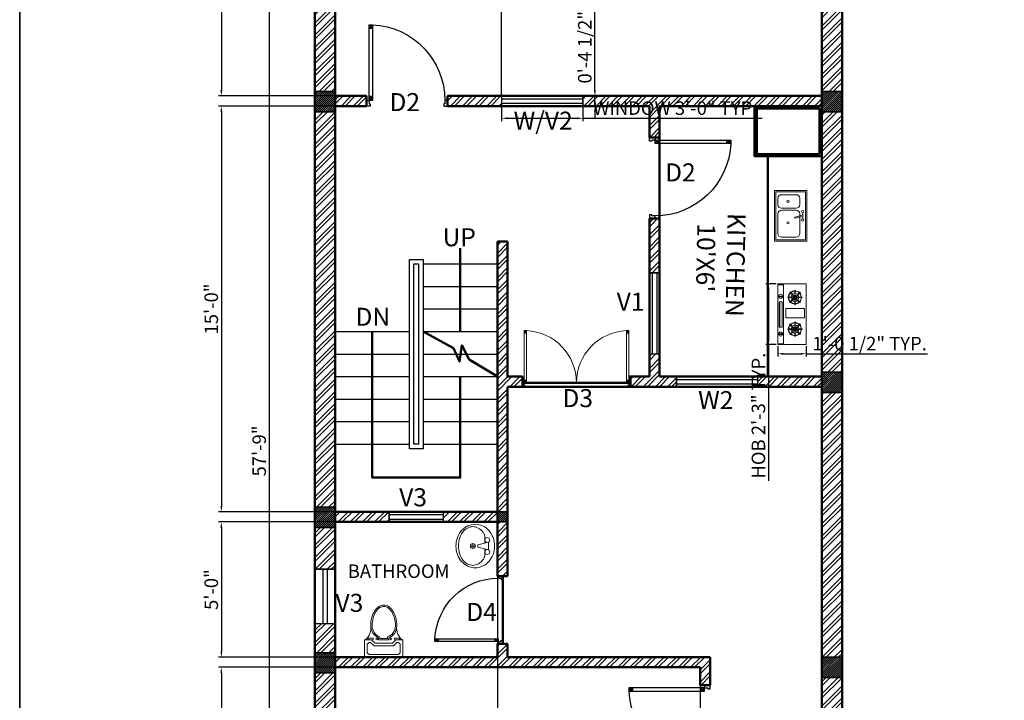
# Model space of a CAD drawing. Units: millimetres. Extents: x 20768 to 23556, y 50760 to 52704.
# Tile 20 of 36: x 20768 to 21205, y 52066 to 52368. Entities that reach past the tile are written whole.
import ezdxf

# ---------------------------------------------------------------- set-up
doc = ezdxf.new("R2010")
doc.units = ezdxf.units.MM
for name, color, linetype, lineweight in [('A-ANNO-DIMS', 2, 'Continuous', 18), ('A-ANNO-TTLB', 7, 'Continuous', 35), ('A-AREA-IDEN', 40, 'Continuous', 18), ('A-DOOR', 3, 'Continuous', 25), ('A-FLOR-STRS', 11, 'Continuous', 25), ('A-FURN', 8, 'Continuous', 18), ('A-GLAZ', 4, 'Continuous', 25), ('A-WALL', 7, 'Continuous', 50), ('A-WALL-PATT', 8, 'Continuous', 13), ('S-ANNO-DIMS', 2, 'Continuous', 18), ('S-COLS', 20, 'Continuous', 35)]:
    doc.layers.add(name, color=color, linetype=linetype, lineweight=lineweight)
doc.styles.get("Standard").update_dxf_attribs({"font": 'arial.ttf'})
doc.dimstyles.new('ISO-25', dxfattribs={"dimtxt": 6, "dimasz": 2.5, "dimexe": 1.25, "dimexo": 0.625, "dimtad": 1, "dimdec": 0, "dimlunit": 3, "dimtxsty": 'Standard', "dimcen": 2.5, "dimadec": 0, "dimazin": 0, "dimtfac": 1, "dimtdec": 0, "dimtmove": 0, "dimatfit": 3, "dimfxl": 1, "dimarcsym": 0})
pattern_1 = [(45, (-81.11126, 0), (-0.449012806, 0.449012806), [])]
pattern_2 = [(45, (-81.1113, 0), (-2.69407684, 2.69407684), []), (45, (-79.3152, 0), (-2.69407684, 2.69407684), [])]

# ---------------------------------------------------------------- blocks, each defined once
blk = doc.blocks.new('Puerta 01')
for p, q in [((-0.7745, -0.0264), (-0.7368, -0.0584)), ((-0.7745, -0.0584), (-0.7368, -0.0264)), ((-0.7368, -0.0584), (-0.7368, -0.0264)), ((-0.028, -0.0584), (-0.0657, -0.0264)), ((-0.028, -0.0264), (-0.0657, -0.0584)), ((-0.0657, -0.0584), (-0.0657, -0.0264))]:
    blk.add_line(p, q)
for points in [[(-0.028, 0), (-0.028, -0.0264), (0.004, -0.0264), (0.004, -0.036), (0.028, -0.036), (0.028, 0)], [(-0.028, -0.0264), (-0.7745, -0.0264), (-0.7745, -0.0584), (-0.028, -0.0584)], [(0.004, -0.7736), (0.004, -0.764), (0.028, -0.764), (0.028, -0.8), (-0.028, -0.8), (-0.028, -0.7736)]]:
    blk.add_lwpolyline(points, close=True)
blk.add_arc((-0.028, -0.0264), 0.7472, 182.45453, 270)
blk = doc.blocks.new('md')
for p, q in [((21281.56, 52416.74), (21282.55, 52415.57)), ((21282.55, 52416.74), (21281.56, 52415.57)), ((21282.55, 52415.57), (21281.56, 52415.57)), ((21327.92, 52416.74), (21326.93, 52415.57)), ((21326.93, 52416.74), (21327.92, 52415.57)), ((21326.93, 52415.57), (21327.92, 52415.57)), ((21282.55, 52393.58), (21281.56, 52394.75)), ((21281.56, 52393.58), (21282.55, 52394.75)), ((21282.55, 52394.75), (21281.56, 52394.75)), ((21326.93, 52393.58), (21327.92, 52394.75)), ((21327.92, 52393.58), (21326.93, 52394.75)), ((21326.93, 52394.75), (21327.92, 52394.75))]:
    blk.add_line(p, q)
for points in [[(21281.56, 52393.58), (21281.56, 52416.74), (21282.55, 52416.74), (21282.55, 52393.58)], [(21327.92, 52393.58), (21327.92, 52416.74), (21326.93, 52416.74), (21326.93, 52393.58)], [(21280.74, 52393.58), (21281.56, 52393.58), (21281.56, 52392.59), (21281.86, 52392.59), (21281.86, 52391.84), (21280.74, 52391.84)], [(21328.74, 52393.58), (21327.92, 52393.58), (21327.92, 52392.59), (21327.62, 52392.59), (21327.62, 52391.84), (21328.74, 52391.84)]]:
    blk.add_lwpolyline(points, close=True)
for centre, start, end in [((21281.56, 52393.58), 0, 87.5455), ((21327.92, 52393.58), 92.4545, 180)]:
    blk.add_arc(centre, 23.18, start, end)
blk = doc.blocks.new('A$C46C9437A')
for p, q in [((0, 416), (0, 1)), ((885, 416), (0, 416)), ((163, 281), (120, 324)), ((167, 285), (124, 328)), ((194, 296), (194, 357)), ((200, 296), (200, 357)), ((228, 284), (271, 326)), ((232, 280), (275, 322)), ((495, 390), (361, 390)), ((361, 390), (361, 118)), ((495, 118), (495, 390)), ((625, 280), (582, 322)), ((628, 284), (586, 326)), ((657, 296), (657, 357)), ((662, 296), (662, 357)), ((690, 285), (733, 328)), ((694, 281), (737, 324)), ((885, 1), (885, 416)), ((152, 255), (91, 255)), ((151, 250), (91, 250)), ((161, 223), (118, 181)), ((164, 219), (121, 177)), ((172, 252), (166, 252)), ((166, 252), (166, 251)), ((166, 251), (172, 251)), ((172, 251), (172, 252)), ((181, 196), (172, 231)), ((194, 205), (194, 145)), ((197, 282), (196, 282)), ((196, 282), (196, 276)), ((196, 276), (197, 276)), ((197, 226), (196, 226)), ((196, 226), (196, 221)), ((196, 221), (197, 221)), ((197, 276), (197, 282)), ((197, 221), (197, 226)), ((200, 205), (200, 145)), ((212, 195), (223, 232)), ((227, 252), (221, 252)), ((221, 252), (221, 251)), ((221, 251), (227, 251)), ((227, 251), (227, 252)), ((227, 217), (270, 174)), ((231, 221), (274, 178)), ((242, 255), (303, 255)), ((242, 250), (303, 250)), ((615, 255), (554, 255)), ((615, 250), (554, 250)), ((626, 221), (583, 178)), ((630, 217), (587, 174)), ((630, 251), (630, 252)), ((630, 252), (636, 252)), ((636, 251), (630, 251)), ((645, 195), (634, 232)), ((636, 252), (636, 251)), ((657, 205), (657, 145)), ((660, 276), (660, 282)), ((660, 282), (661, 282)), ((661, 276), (660, 276)), ((660, 221), (660, 226)), ((660, 226), (661, 226)), ((661, 221), (660, 221)), ((661, 282), (661, 276)), ((661, 226), (661, 221)), ((662, 205), (662, 145)), ((676, 196), (685, 231)), ((685, 251), (685, 252)), ((685, 252), (691, 252)), ((691, 251), (685, 251)), ((691, 252), (691, 251)), ((693, 219), (736, 177)), ((696, 223), (739, 181)), ((705, 255), (766, 255)), ((706, 250), (766, 250)), ((0, 82), (885, 82)), ((0, 1), (885, 1)), ((12, 0), (12, 82)), ((185, 71), (177, 71)), ((177, 71), (177, 16)), ((177, 16), (185, 16)), ((185, 16), (185, 71)), ((629, 65), (261, 65)), ((261, 65), (261, 21)), ((629, 33), (261, 33)), ((261, 21), (629, 21)), ((361, 118), (495, 118)), ((629, 21), (629, 65)), ((736, 71), (728, 71)), ((728, 71), (728, 16)), ((728, 16), (736, 16)), ((736, 16), (736, 71)), ((872, 0), (872, 82))]:
    blk.add_line(p, q)
for centre, radius in [((197, 251), 32.5), ((197, 251), 30.7), ((174, 252), 2.11), ((181, 267), 2.11), ((180, 236), 2.11), ((196, 252), 14.5), ((196, 252), 12.7), ((196, 252), 4.75), ((197, 274), 2.11), ((197, 228), 2.11), ((212, 267), 2.11), ((212, 236), 2.11), ((219, 252), 2.11), ((660, 251), 32.5), ((660, 251), 30.7), ((638, 252), 2.11), ((645, 267), 2.11), ((645, 236), 2.11), ((661, 252), 14.5), ((661, 252), 12.7), ((661, 252), 4.75), ((660, 274), 2.11), ((660, 228), 2.11), ((676, 267), 2.11), ((677, 236), 2.11), ((683, 252), 2.11), ((180, 44), 29), ((731, 44), 29)]:
    blk.add_circle(centre, radius)
for centre, radius, start, end in [((197, 251), 94.6, 136.5182, 177.4268), ((197, 251), 91, 136.5783, 177.3249), ((197, 251), 106, 133.4332, 136.3568), ((197, 251), 94.6, 91.4483, 133.2468), ((197, 251), 91, 91.5056, 133.1774), ((197, 251), 57.2, 92.3972, 175.7393), ((197, 239), 118, 88.3708, 91.2943), ((197, 251), 45.5, 86.2077, 93.012), ((197, 251), 94.6, 45.53, 88.1769), ((197, 251), 91, 45.5509, 88.1047), ((197, 251), 57.2, 45.877, 86.9821), ((197, 251), 57.2, 4.2607, 40.4593), ((197, 251), 91, 2.6751, 42.1494), ((197, 251), 94.6, 2.5732, 42.2579), ((197, 251), 106, 42.5497, 45.4736), ((660, 251), 94.6, 137.7421, 177.4268), ((660, 251), 91, 137.8506, 177.3249), ((660, 251), 106, 134.5264, 137.4503), ((660, 251), 94.6, 91.8231, 134.47), ((660, 251), 91, 91.8953, 134.4491), ((660, 251), 57.2, 139.5407, 175.7393), ((660, 251), 57.2, 93.0179, 134.123), ((660, 239), 118, 88.7057, 91.6292), ((660, 251), 45.5, 86.988, 93.7923), ((660, 251), 94.6, 46.7532, 88.5517), ((660, 251), 91, 46.8226, 88.4944), ((660, 251), 57.2, 4.2607, 87.6028), ((660, 251), 91, 2.6751, 43.4217), ((660, 251), 94.6, 2.5732, 43.4818), ((660, 251), 106, 43.6432, 46.5668), ((209, 250), 118, 177.7006, 180.3321), ((197, 251), 94.6, 180.6987, 221.1963), ((197, 251), 91, 180.7263, 221.0455), ((197, 251), 106, 221.6012, 224.5264), ((197, 251), 94.6, 224.47, 268.5517), ((197, 251), 91, 224.4491, 268.4944), ((197, 251), 57.2, 181.1563, 218.6973), ((197, 251), 45.5, 174.6446, 181.4526), ((197, 251), 57.2, 224.123, 267.6028), ((197, 251), 45.5, 217.0728, 223.8982), ((197, 251), 45.5, 131.3533, 138.1575), ((197, 251), 45.5, 266.988, 273.7923), ((197, 251), 106, 268.7057, 271.6292), ((197, 251), 57.2, 273.0179, 312.4871), ((197, 251), 91, 271.8953, 313.4217), ((197, 251), 94.6, 271.8231, 313.4818), ((197, 251), 45.5, 311.8425, 318.6467), ((197, 251), 45.5, 39.2922, 46.1018), ((197, 251), 57.2, 317.9021, 358.8437), ((197, 251), 45.5, 358.5474, 5.3554), ((197, 251), 91, 316.8226, 359.2737), ((197, 251), 94.6, 316.7532, 359.3013), ((197, 251), 106, 313.6432, 316.5668), ((197, 251), 106, 359.3756, 2.2994), ((660, 251), 106, 177.7006, 180.6244), ((660, 251), 94.6, 180.6987, 223.2468), ((660, 251), 91, 180.7263, 223.1774), ((660, 251), 106, 223.4332, 226.3568), ((660, 251), 94.6, 226.5182, 268.1769), ((660, 251), 91, 226.5783, 268.1047), ((660, 251), 57.2, 181.1563, 222.0979), ((660, 251), 45.5, 174.6446, 181.4526), ((660, 251), 57.2, 227.5129, 266.9821), ((660, 251), 45.5, 133.8982, 140.7078), ((660, 251), 45.5, 221.3533, 228.1575), ((660, 251), 45.5, 266.2077, 273.012), ((660, 251), 106, 268.3708, 271.2943), ((660, 251), 57.2, 272.3972, 315.877), ((660, 251), 91, 271.5056, 315.5509), ((660, 251), 94.6, 271.4483, 315.53), ((660, 251), 45.5, 41.8425, 48.6467), ((660, 251), 45.5, 316.1018, 322.9272), ((660, 251), 45.5, 358.5474, 5.3554), ((660, 251), 57.2, 321.3027, 358.8437), ((660, 251), 91, 318.9545, 359.2737), ((660, 251), 94.6, 318.8037, 359.3013), ((660, 251), 106, 315.4736, 318.3988), ((648, 250), 118, 359.6679, 2.2994)]:
    blk.add_arc(centre, radius, start, end)
blk = doc.blocks.new('A$C42714C99')
for p, q in [((0, 445), (0, 5)), ((695, 450), (5, 450)), ((20, 430), (20, 20)), ((680, 430), (20, 430)), ((680, 20), (680, 430)), ((700, 5), (700, 445)), ((57, 99), (57, 302)), ((107, 352), (195, 352)), ((245, 302), (245, 99)), ((273, 99), (273, 302)), ((304, 393), (393, 393)), ((323, 352), (595, 352)), ((335, 393), (369, 287)), ((360, 393), (382, 288)), ((645, 302), (645, 99)), ((5, 0), (695, 0)), ((20, 20), (680, 20)), ((195, 49), (107, 49)), ((595, 49), (323, 49))]:
    blk.add_line(p, q)
for centre in [(289, 393), (408, 393), (148, 188), (446, 188)]:
    blk.add_circle(centre, 15.1)
for centre, radius, start, end in [((5, 445), 5, 90, 180), ((695, 445), 5, 0, 90), ((107, 302), 50, 90, 180), ((195, 302), 50, 0, 90), ((323, 302), 50, 90, 180), ((375, 290), 6.89, 207.5958, 343.0526), ((595, 302), 50, 0, 90), ((5, 5), 5, 180, 270), ((1, 1), 1, 180, 270), ((107, 99), 50, 180, 270), ((195, 99), 50, 270, 0), ((323, 99), 50, 180, 270), ((595, 99), 50, 270, 0), ((695, 5), 5, 270, 0), ((699, 1), 1, 270, 0)]:
    blk.add_arc(centre, radius, start, end)
blk = doc.blocks.new('A$C00DA51E9')
blk.add_blockref('A$C42714C99', (0, 0))
blk = doc.blocks.new('A$C0E746A5D')
for p, q in [((0.105, 0.332), (0.105, 0.269)), ((0.066, 0.276), (0.066, 0.197)), ((0.079, 0.276), (0.184, 0.25)), ((0.184, 0.223), (0.079, 0.197)), ((0.184, 0.25), (0.184, 0.223)), ((0.21, 0.237), (0.263, 0.237)), ((0.237, 0.263), (0.237, 0.21)), ((0.105, 0.204), (0.105, 0.141))]:
    blk.add_line(p, q)
for centre in [(0.079, 0.302), (0.237, 0.237), (0.079, 0.171)]:
    blk.add_circle(centre, 0.0263)
for centre, radius, start, end in [((0.221, 0.262), 0.214, 114.9851, 138.3665), ((0.261, 0.284), 0.17, 118.9112, 147.7402), ((0.21, 0.286), 0.188, 90, 114.9851), ((0.237, 0.327), 0.12, 90, 118.9112), ((0.21, 0.286), 0.188, 65.0149, 90), ((0.237, 0.327), 0.12, 61.0888, 90), ((0.199, 0.262), 0.214, 41.6335, 65.0149), ((0.213, 0.284), 0.17, 36.8699, 61.0888), ((0.266, 0.237), 0.266, 159.7868, 180), ((0.239, 0.247), 0.237, 138.3665, 159.7868), ((0.184, 0.332), 0.0789, 147.7402, 180), ((0.175, 0.255), 0.217, 17.2579, 36.8699), ((0.182, 0.247), 0.237, 20.2132, 41.6335), ((0.155, 0.237), 0.266, 0, 20.2132), ((0.266, 0.237), 0.266, 180, 200.2132), ((0.115, 0.237), 0.279, 0, 17.2579), ((0.115, 0.237), 0.279, 342.7421, 0), ((0.155, 0.237), 0.266, 339.7868, 360), ((0.239, 0.227), 0.237, 200.2132, 221.6335), ((0.184, 0.141), 0.0789, 180, 213.9045), ((0.175, 0.218), 0.217, 323.1301, 342.7421), ((0.182, 0.227), 0.237, 318.3665, 339.7868), ((0.221, 0.211), 0.214, 221.6335, 245.0149), ((0.299, 0.218), 0.217, 213.9045, 216.8699), ((0.261, 0.19), 0.17, 216.8699, 241.0888), ((0.21, 0.188), 0.188, 245.0149, 270), ((0.237, 0.146), 0.12, 241.0888, 270), ((0.21, 0.188), 0.188, 270, 294.9851), ((0.237, 0.146), 0.12, 270, 298.9112), ((0.199, 0.211), 0.214, 294.9851, 318.3665), ((0.213, 0.19), 0.17, 298.9112, 323.1301)]:
    blk.add_arc(centre, radius, start, end)
blk = doc.blocks.new('A$C098B081F')
for p, q in [((559, 762), (0, 762)), ((0, 762), (0, 508)), ((63, 724), (38, 698)), ((495, 724), (63, 724)), ((521, 698), (495, 724)), ((559, 762), (559, 508)), ((38, 698), (38, 571)), ((137, 597), (86, 546)), ((422, 597), (137, 597)), ((422, 597), (473, 546)), ((521, 698), (521, 571)), ((0, 508), (13, 508)), ((13, 508), (102, 508)), ((38, 571), (63, 546)), ((51, 508), (51, 483)), ((51, 508), (102, 508)), ((51, 483), (114, 483)), ((63, 546), (86, 546)), ((152, 559), (102, 508)), ((114, 508), (102, 508)), ((406, 559), (152, 559)), ((203, 508), (203, 479)), ((203, 508), (356, 508)), ((223, 488), (223, 466)), ((223, 488), (336, 488)), ((336, 488), (336, 466)), ((356, 508), (356, 479)), ((406, 559), (457, 508)), ((444, 508), (457, 508)), ((508, 483), (444, 483)), ((508, 508), (457, 508)), ((495, 546), (473, 546)), ((495, 546), (521, 571)), ((508, 508), (546, 508)), ((508, 508), (508, 483)), ((559, 508), (546, 508))]:
    blk.add_line(p, q)
for centre in [(178, 495), (381, 495)]:
    blk.add_circle(centre, 12.7)
for centre, radius, start, end in [((-137, 336), 228, 352.2011, 48.911), ((279, 305), 190, 113.5782, 180), ((279, 305), 170, 109.2456, 180), ((114, 495), 12.7, 270, 90), ((279, 305), 170, 0, 70.7544), ((279, 305), 190, 0, 66.4218), ((444, 495), 12.7, 90, 270), ((696, 336), 228, 131.089, 187.7989), ((575, 305), 486, 180, 194.5143), ((575, 305), 466, 180, 194.5143), ((-16, 305), 466, 345.4857, 360), ((-16, 305), 486, 345.4857, 360), ((429, 267), 335, 194.5143, 212.0054), ((429, 267), 315, 194.5143, 212.0054), ((130, 267), 315, 327.9946, 345.4857), ((130, 267), 335, 327.9946, 345.4857), ((337, 210), 227, 212.0054, 236.4659), ((337, 210), 207, 212.0054, 236.4659), ((279, 122), 122, 236.4659, 270), ((279, 122), 102, 236.4659, 270), ((279, 122), 102, 270, 303.5341), ((279, 122), 122, 270, 303.5341), ((222, 210), 207, 303.5341, 327.9946), ((222, 210), 227, 303.5341, 327.9946)]:
    blk.add_arc(centre, radius, start, end)
blk = doc.blocks.new('*D108')
at = {"layer": 'A-ANNO-DIMS', "color": 0, "lineweight": -2, "transparency": 16777216}
for p, q in [((20898.51, 52522.9), (20877.66, 52522.9)), ((20878.91, 52520.4), (20878.91, 51832.4)), ((20898.51, 51829.9), (20877.66, 51829.9))]:
    blk.add_line(p, q, dxfattribs=at)
at = {"layer": 'A-ANNO-DIMS', "color": 0, "transparency": 16777216}
for points in [[(20878.49, 52520.4), (20879.33, 52520.4), (20878.91, 52522.9)], [(20878.49, 51832.4), (20879.33, 51832.4), (20878.91, 51829.9)]]:
    blk.add_solid(points, dxfattribs=at)
at = {"layer": 'Defpoints', "color": 0, "transparency": 16777216}
for p in [(20899.14, 52522.9), (20878.91, 51829.9), (20899.14, 51829.9)]:
    blk.add_point(p, dxfattribs=at)
at = {"layer": 'A-ANNO-DIMS', "color": 0, "transparency": 16777216, "insert": (20875.22, 52176.4), "char_height": 6, "attachment_point": 5, "rotation": 90}
blk.add_mtext('57\'-9"', dxfattribs=at)
blk = doc.blocks.new('COL-PLAN')
blk.add_line((0, 9), (9, 9))
blk.add_lwpolyline([(9, 9), (0, 9), (0, 0), (9, 0)], close=True)
blk = doc.blocks.new('WIN-PLAN-A')
blk.add_line((36, 4.5), (36, 0))
blk.add_lwpolyline([(36, 4.5), (0, 4.5), (0, 0), (36, 0)], close=True)
blk = doc.blocks.new('WIN-PLAN-B')
blk.add_line((0, 4.5), (0, 0))
blk.add_lwpolyline([(0, 4.5), (24, 4.5), (24, 0), (0, 0)], close=True)
blk = doc.blocks.new('WIN-PLAN-D')
blk.add_line((0, 24), (9, 24))
blk.add_lwpolyline([(9, 24), (0, 24), (0, 0), (9, 0)], close=True)
blk = doc.blocks.new('*D175')
at = {"layer": 'Defpoints', "color": 0, "transparency": 16777216}
for p in [(20982.04, 52329.4), (21018.04, 52329.4), (21018.04, 52324)]:
    blk.add_point(p, dxfattribs=at)
at = {"layer": 'S-ANNO-DIMS', "color": 0, "lineweight": -2, "transparency": 16777216}
for p, q in [((20982.04, 52328.77), (20982.04, 52322.75)), ((21018.04, 52328.77), (21018.04, 52322.75)), ((20984.54, 52324), (21015.54, 52324)), ((21018.04, 52324), (21097.71, 52324))]:
    blk.add_line(p, q, dxfattribs=at)
at = {"layer": 'S-ANNO-DIMS', "color": 0, "transparency": 16777216}
for points in [[(20984.54, 52324.41), (20984.54, 52323.58), (20982.04, 52324)], [(21015.54, 52324.41), (21015.54, 52323.58), (21018.04, 52324)]]:
    blk.add_solid(points, dxfattribs=at)
at = {"layer": 'S-ANNO-DIMS', "color": 0, "transparency": 16777216, "insert": (21059.13, 52327.73), "char_height": 6, "attachment_point": 5}
blk.add_mtext('WINDOW 3\'-0" TYP.', dxfattribs=at)
blk = doc.blocks.new('*D176')
at = {"layer": 'Defpoints', "color": 0, "transparency": 16777216}
for p in [(21018.04, 52333.9), (21023.44, 52333.9), (21018.04, 52329.4)]:
    blk.add_point(p, dxfattribs=at)
at = {"layer": 'S-ANNO-DIMS', "color": 0, "lineweight": -2, "transparency": 16777216}
for p, q in [((21023.44, 52336.4), (21023.44, 52390.7)), ((21018.66, 52333.9), (21024.69, 52333.9)), ((21023.44, 52329.4), (21023.44, 52333.9)), ((21018.66, 52329.4), (21024.69, 52329.4)), ((21023.44, 52326.9), (21023.44, 52324.4))]:
    blk.add_line(p, q, dxfattribs=at)
at = {"layer": 'S-ANNO-DIMS', "color": 0, "transparency": 16777216}
for points in [[(21023.02, 52336.4), (21023.86, 52336.4), (21023.44, 52333.9)], [(21023.02, 52326.9), (21023.86, 52326.9), (21023.44, 52329.4)]]:
    blk.add_solid(points, dxfattribs=at)
at = {"layer": 'S-ANNO-DIMS', "color": 0, "transparency": 16777216, "insert": (21019.71, 52364.8), "char_height": 6, "attachment_point": 5, "rotation": 90}
blk.add_mtext('0\'-4 1/2" TYP.', dxfattribs=at)
blk = doc.blocks.new('*D193')
at = {"layer": 'Defpoints', "color": 0, "transparency": 16777216}
for p in [(21104.57, 52250.54), (21100.52, 52223.57), (21104.57, 52223.57)]:
    blk.add_point(p, dxfattribs=at)
at = {"layer": 'S-ANNO-DIMS', "color": 0, "lineweight": -2, "transparency": 16777216}
for p, q in [((21103.94, 52250.54), (21099.27, 52250.54)), ((21100.52, 52248.04), (21100.52, 52226.07)), ((21103.94, 52223.57), (21099.27, 52223.57)), ((21100.52, 52223.57), (21100.52, 52163.08))]:
    blk.add_line(p, q, dxfattribs=at)
at = {"layer": 'S-ANNO-DIMS', "color": 0, "transparency": 16777216}
for points in [[(21100.11, 52248.04), (21100.94, 52248.04), (21100.52, 52250.54)], [(21100.11, 52226.07), (21100.94, 52226.07), (21100.52, 52223.57)]]:
    blk.add_solid(points, dxfattribs=at)
at = {"layer": 'S-ANNO-DIMS', "color": 0, "transparency": 16777216, "insert": (21096.79, 52192.08), "char_height": 6, "attachment_point": 5, "rotation": 90}
blk.add_mtext('HOB 2\'-3" TYP.', dxfattribs=at)
blk = doc.blocks.new('*D194')
at = {"layer": 'Defpoints', "color": 0, "transparency": 16777216}
for p in [(21104.57, 52223.57), (21117.26, 52223.57), (21117.26, 52219.53)]:
    blk.add_point(p, dxfattribs=at)
at = {"layer": 'S-ANNO-DIMS', "color": 0, "lineweight": -2, "transparency": 16777216}
for p, q in [((21104.57, 52222.95), (21104.57, 52218.28)), ((21117.26, 52222.95), (21117.26, 52218.28)), ((21107.07, 52219.53), (21114.76, 52219.53)), ((21117.26, 52219.53), (21171, 52219.53))]:
    blk.add_line(p, q, dxfattribs=at)
at = {"layer": 'S-ANNO-DIMS', "color": 0, "transparency": 16777216}
for points in [[(21107.07, 52219.94), (21107.07, 52219.11), (21104.57, 52219.53)], [(21114.76, 52219.94), (21114.76, 52219.11), (21117.26, 52219.53)]]:
    blk.add_solid(points, dxfattribs=at)
at = {"layer": 'S-ANNO-DIMS', "color": 0, "transparency": 16777216, "insert": (21145.38, 52223.25), "char_height": 6, "attachment_point": 5}
blk.add_mtext('1\'-0 1/2" TYP.', dxfattribs=at)
blk = doc.blocks.new('*D201')
at = {"layer": 'Defpoints', "color": 0, "transparency": 16777216}
for p in [(20908.14, 52513.9), (20857.64, 52333.9), (20908.14, 52333.9)]:
    blk.add_point(p, dxfattribs=at)
at = {"layer": 'S-ANNO-DIMS', "color": 0, "lineweight": -2, "transparency": 16777216}
for p, q in [((20907.51, 52513.9), (20856.39, 52513.9)), ((20857.64, 52511.4), (20857.64, 52336.4)), ((20907.51, 52333.9), (20856.39, 52333.9))]:
    blk.add_line(p, q, dxfattribs=at)
at = {"layer": 'S-ANNO-DIMS', "color": 0, "transparency": 16777216}
for points in [[(20857.22, 52511.4), (20858.06, 52511.4), (20857.64, 52513.9)], [(20857.22, 52336.4), (20858.06, 52336.4), (20857.64, 52333.9)]]:
    blk.add_solid(points, dxfattribs=at)
at = {"layer": 'S-ANNO-DIMS', "color": 0, "transparency": 16777216, "insert": (20853.95, 52423.9), "char_height": 6, "attachment_point": 5, "rotation": 90}
blk.add_mtext('15\'-0"', dxfattribs=at)
blk = doc.blocks.new('*D202')
at = {"layer": 'Defpoints', "color": 0, "transparency": 16777216}
for p in [(20908.14, 52329.4), (20857.64, 52149.4), (20908.14, 52149.4)]:
    blk.add_point(p, dxfattribs=at)
at = {"layer": 'S-ANNO-DIMS', "color": 0, "lineweight": -2, "transparency": 16777216}
for p, q in [((20907.51, 52329.4), (20856.39, 52329.4)), ((20857.64, 52326.9), (20857.64, 52151.9)), ((20907.51, 52149.4), (20856.39, 52149.4))]:
    blk.add_line(p, q, dxfattribs=at)
at = {"layer": 'S-ANNO-DIMS', "color": 0, "transparency": 16777216}
for points in [[(20857.22, 52326.9), (20858.06, 52326.9), (20857.64, 52329.4)], [(20857.22, 52151.9), (20858.06, 52151.9), (20857.64, 52149.4)]]:
    blk.add_solid(points, dxfattribs=at)
at = {"layer": 'S-ANNO-DIMS', "color": 0, "transparency": 16777216, "insert": (20853.95, 52239.4), "char_height": 6, "attachment_point": 5, "rotation": 90}
blk.add_mtext('15\'-0"', dxfattribs=at)
blk = doc.blocks.new('*D203')
at = {"layer": 'Defpoints', "color": 0, "transparency": 16777216}
for p in [(20908.14, 52144.9), (20857.64, 52084.9), (20908.14, 52084.9)]:
    blk.add_point(p, dxfattribs=at)
at = {"layer": 'S-ANNO-DIMS', "color": 0, "lineweight": -2, "transparency": 16777216}
for p, q in [((20907.51, 52144.9), (20856.39, 52144.9)), ((20857.64, 52142.4), (20857.64, 52087.4)), ((20907.51, 52084.9), (20856.39, 52084.9))]:
    blk.add_line(p, q, dxfattribs=at)
at = {"layer": 'S-ANNO-DIMS', "color": 0, "transparency": 16777216}
for points in [[(20857.22, 52142.4), (20858.06, 52142.4), (20857.64, 52144.9)], [(20857.22, 52087.4), (20858.06, 52087.4), (20857.64, 52084.9)]]:
    blk.add_solid(points, dxfattribs=at)
at = {"layer": 'S-ANNO-DIMS', "color": 0, "transparency": 16777216, "insert": (20853.95, 52114.9), "char_height": 6, "attachment_point": 5, "rotation": 90}
blk.add_mtext('5\'-0"', dxfattribs=at)
blk = doc.blocks.new('*D204')
at = {"layer": 'Defpoints', "color": 0, "transparency": 16777216}
for p in [(20908.14, 52080.4), (20857.64, 51900.4), (20908.14, 51900.4)]:
    blk.add_point(p, dxfattribs=at)
at = {"layer": 'S-ANNO-DIMS', "color": 0, "lineweight": -2, "transparency": 16777216}
for p, q in [((20907.51, 52080.4), (20856.39, 52080.4)), ((20857.64, 52077.9), (20857.64, 51902.9)), ((20907.51, 51900.4), (20856.39, 51900.4))]:
    blk.add_line(p, q, dxfattribs=at)
at = {"layer": 'S-ANNO-DIMS', "color": 0, "transparency": 16777216}
for points in [[(20857.22, 52077.9), (20858.06, 52077.9), (20857.64, 52080.4)], [(20857.22, 51902.9), (20858.06, 51902.9), (20857.64, 51900.4)]]:
    blk.add_solid(points, dxfattribs=at)
at = {"layer": 'S-ANNO-DIMS', "color": 0, "transparency": 16777216, "insert": (20853.95, 51990.4), "char_height": 6, "attachment_point": 5, "rotation": 90}
blk.add_mtext('15\'-0"', dxfattribs=at)
blk = doc.blocks.new('*D206')
at = {"layer": 'Defpoints', "color": 0, "transparency": 16777216}
for p in [(20908.14, 52144.9), (20980.14, 52144.9), (20980.14, 51776.4)]:
    blk.add_point(p, dxfattribs=at)
at = {"layer": 'S-ANNO-DIMS', "color": 0, "lineweight": -2, "transparency": 16777216}
for p, q in [((20908.14, 52144.27), (20908.14, 51775.15)), ((20980.14, 52144.27), (20980.14, 51775.15)), ((20910.64, 51776.4), (20977.64, 51776.4))]:
    blk.add_line(p, q, dxfattribs=at)
at = {"layer": 'S-ANNO-DIMS', "color": 0, "transparency": 16777216}
for points in [[(20910.64, 51776.81), (20910.64, 51775.98), (20908.14, 51776.4)], [(20977.64, 51776.81), (20977.64, 51775.98), (20980.14, 51776.4)]]:
    blk.add_solid(points, dxfattribs=at)
at = {"layer": 'S-ANNO-DIMS', "color": 0, "transparency": 16777216, "insert": (20944.14, 51780.09), "char_height": 6, "attachment_point": 5}
blk.add_mtext('6\'-0"', dxfattribs=at)
blk = doc.blocks.new('*D207')
at = {"layer": 'Defpoints', "color": 0, "transparency": 16777216}
for p in [(20908.14, 52080.4), (21070.14, 52080.4), (21070.14, 51776.4)]:
    blk.add_point(p, dxfattribs=at)
at = {"layer": 'S-ANNO-DIMS', "color": 0, "lineweight": -2, "transparency": 16777216}
for p, q in [((20908.14, 52079.77), (20908.14, 51775.15)), ((21070.14, 52079.77), (21070.14, 51775.15)), ((20910.64, 51776.4), (21067.64, 51776.4))]:
    blk.add_line(p, q, dxfattribs=at)
at = {"layer": 'S-ANNO-DIMS', "color": 0, "transparency": 16777216}
for points in [[(20910.64, 51776.81), (20910.64, 51775.98), (20908.14, 51776.4)], [(21067.64, 51776.81), (21067.64, 51775.98), (21070.14, 51776.4)]]:
    blk.add_solid(points, dxfattribs=at)
at = {"layer": 'S-ANNO-DIMS', "color": 0, "transparency": 16777216, "insert": (20989.14, 51780.09), "char_height": 6, "attachment_point": 5}
blk.add_mtext('13\'-6"', dxfattribs=at)
blk = doc.blocks.new('*D209')
at = {"layer": 'Defpoints', "color": 0, "transparency": 16777216}
for p in [(20982.04, 52564.4), (20908.14, 52333.9), (20982.04, 52333.9)]:
    blk.add_point(p, dxfattribs=at)
at = {"layer": 'S-ANNO-DIMS', "color": 0, "lineweight": -2, "transparency": 16777216}
for p, q in [((20908.14, 52334.52), (20908.14, 52565.65)), ((20910.64, 52564.4), (20979.54, 52564.4)), ((20982.04, 52334.52), (20982.04, 52565.65))]:
    blk.add_line(p, q, dxfattribs=at)
at = {"layer": 'S-ANNO-DIMS', "color": 0, "transparency": 16777216}
for points in [[(20910.64, 52564.81), (20910.64, 52563.98), (20908.14, 52564.4)], [(20979.54, 52564.81), (20979.54, 52563.98), (20982.04, 52564.4)]]:
    blk.add_solid(points, dxfattribs=at)
at = {"layer": 'S-ANNO-DIMS', "color": 0, "transparency": 16777216, "insert": (20945.09, 52568.09), "char_height": 6, "attachment_point": 5}
blk.add_mtext('6\'-2"', dxfattribs=at)

msp = doc.modelspace()

# ---------------------------------------------------------------- hatches: boundary and pattern name
at = {"layer": 'A-WALL-PATT'}
h = msp.add_hatch(dxfattribs=at)
h.set_pattern_fill('ANSI32', color=256, scale=0.4)
h.set_pattern_definition(pattern_2)
h.paths.add_polyline_path([(20908.14, 52513.9), (20899.14, 52513.9), (20899.14, 52335.9), (20908.14, 52335.9)])
h = msp.add_hatch(dxfattribs=at)
h.set_pattern_fill('ANSI32', color=256, scale=0.4)
h.set_pattern_definition(pattern_2)
h.paths.add_polyline_path([(21133.14, 52513.9), (21124.14, 52513.9), (21124.14, 52335.9), (21133.14, 52335.9)])
h = msp.add_hatch(dxfattribs=at)
h.set_pattern_fill('ANSI31', color=256, scale=0.2)
h.set_pattern_definition(pattern_1)
h.paths.add_polyline_path([(20908.14, 52335.9), (20899.14, 52335.9), (20899.14, 52326.9), (20908.14, 52326.9)])
h = msp.add_hatch(dxfattribs=at)
h.set_pattern_fill('ANSI31', color=256, scale=0.2)
h.set_pattern_definition(pattern_1)
h.paths.add_polyline_path([(21133.14, 52335.9), (21124.14, 52335.9), (21124.14, 52326.9), (21133.14, 52326.9)])
h = msp.add_hatch(dxfattribs=at)
h.set_pattern_fill('ANSI32', color=256, scale=0.4)
h.set_pattern_definition(pattern_2)
h.paths.add_polyline_path([(20922.04, 52333.9), (20908.14, 52333.9), (20908.14, 52329.4), (20922.04, 52329.4), (20922.04, 52331.92)])
h = msp.add_hatch(dxfattribs=at)
h.set_pattern_fill('ANSI32', color=256, scale=0.4)
h.set_pattern_definition(pattern_2)
h.paths.add_polyline_path([(20982.04, 52333.9), (20958.04, 52333.9), (20958.04, 52329.4), (20982.04, 52329.4)])
h = msp.add_hatch(dxfattribs=at)
h.set_pattern_fill('ANSI32', color=256, scale=0.4)
h.set_pattern_definition(pattern_2)
h.paths.add_polyline_path([(21124.14, 52333.9), (21018.04, 52333.9), (21018.04, 52329.4), (21047.64, 52329.4), (21047.64, 52315.5), (21050.16, 52315.5), (21052.14, 52315.5), (21052.14, 52329.4), (21124.14, 52329.4)])
h = msp.add_hatch(dxfattribs=at)
h.set_pattern_fill('ANSI32', color=256, scale=0.4)
h.set_pattern_definition(pattern_2)
h.paths.add_polyline_path([(20908.14, 52326.9), (20899.14, 52326.9), (20899.14, 52151.4), (20908.14, 52151.4)])
h = msp.add_hatch(dxfattribs=at)
h.set_pattern_fill('ANSI32', color=256, scale=0.4)
h.set_pattern_definition(pattern_2)
h.paths.add_polyline_path([(21133.14, 52326.9), (21124.14, 52326.9), (21124.14, 52307.13), (21124.14, 52211.4), (21133.14, 52211.4)])
h = msp.add_hatch(dxfattribs=at)
h.set_pattern_fill('ANSI32', color=256, scale=0.4)
h.set_pattern_definition(pattern_2)
h.paths.add_polyline_path([(21052.14, 52279.5), (21047.64, 52279.5), (21047.64, 52255.5), (21052.14, 52255.5)])
h = msp.add_hatch(dxfattribs=at)
h.set_pattern_fill('ANSI32', color=256, scale=0.4)
h.set_pattern_definition(pattern_2)
h.paths.add_polyline_path([(20991.24, 52206.63), (20991.24, 52209.4), (20984.64, 52209.4), (20984.64, 52269.4), (20980.14, 52269.4), (20980.14, 52149.4), (20984.64, 52149.4), (20984.64, 52204.9), (20991.24, 52204.9)])
h = msp.add_hatch(dxfattribs=at)
h.set_pattern_fill('ANSI32', color=256, scale=0.4)
h.set_pattern_definition(pattern_2)
h.paths.add_polyline_path([(21059.64, 52209.4), (21052.14, 52209.4), (21052.14, 52219.5), (21047.64, 52219.5), (21047.64, 52209.4), (21039.24, 52209.4), (21039.24, 52204.9), (21059.64, 52204.9)])
h = msp.add_hatch(dxfattribs=at)
h.set_pattern_fill('ANSI32', color=256, scale=0.4)
h.set_pattern_definition(pattern_2)
h.paths.add_polyline_path([(21124.14, 52209.4), (21095.64, 52209.4), (21095.64, 52204.9), (21124.14, 52204.9)])
h = msp.add_hatch(dxfattribs=at)
h.set_pattern_fill('ANSI31', color=256, scale=0.2)
h.set_pattern_definition(pattern_1)
h.paths.add_polyline_path([(21133.14, 52211.4), (21124.14, 52211.4), (21124.14, 52202.4), (21133.14, 52202.4)])
h = msp.add_hatch(dxfattribs=at)
h.set_pattern_fill('ANSI32', color=256, scale=0.4)
h.set_pattern_definition(pattern_2)
h.paths.add_polyline_path([(21133.14, 52202.4), (21124.14, 52202.4), (21124.14, 52084.9), (21133.14, 52084.9)])
h = msp.add_hatch(dxfattribs=at)
h.set_pattern_fill('ANSI31', color=256, scale=0.2)
h.set_pattern_definition(pattern_1)
h.paths.add_polyline_path([(20908.14, 52151.4), (20899.14, 52151.4), (20899.14, 52142.4), (20908.14, 52142.4)])
h = msp.add_hatch(dxfattribs=at)
h.set_pattern_fill('ANSI32', color=256, scale=0.4)
h.set_pattern_definition(pattern_2)
h.paths.add_polyline_path([(20932.14, 52149.4), (20908.14, 52149.4), (20908.14, 52144.9), (20932.14, 52144.9)])
h = msp.add_hatch(dxfattribs=at)
h.set_pattern_fill('ANSI32', color=256, scale=0.4)
h.set_pattern_definition(pattern_2)
h.paths.add_polyline_path([(20980.14, 52149.4), (20956.14, 52149.4), (20956.14, 52144.9), (20980.14, 52144.9)])
h = msp.add_hatch(dxfattribs=at)
h.set_pattern_fill('ANSI31', color=256, scale=0.2)
h.set_pattern_definition(pattern_1)
h.paths.add_polyline_path([(20984.64, 52149.4), (20980.14, 52149.4), (20980.14, 52144.9), (20984.64, 52144.9)])
h = msp.add_hatch(dxfattribs=at)
h.set_pattern_fill('ANSI32', color=256, scale=0.4)
h.set_pattern_definition(pattern_2)
h.paths.add_polyline_path([(20908.14, 52142.4), (20899.14, 52142.4), (20899.14, 52123.9), (20908.14, 52123.9)])
h = msp.add_hatch(dxfattribs=at)
h.set_pattern_fill('ANSI32', color=256, scale=0.4)
h.set_pattern_definition(pattern_2)
h.paths.add_polyline_path([(20984.64, 52144.9), (20980.14, 52144.9), (20980.14, 52120.9), (20984.64, 52120.9)])
h = msp.add_hatch(dxfattribs=at)
h.set_pattern_fill('ANSI32', color=256, scale=0.4)
h.set_pattern_definition(pattern_2)
h.paths.add_polyline_path([(20908.14, 52099.9), (20899.14, 52099.9), (20899.14, 52086.9), (20908.14, 52086.9)])
h = msp.add_hatch(dxfattribs=at)
h.set_pattern_fill('ANSI32', color=256, scale=0.4)
h.set_pattern_definition(pattern_2)
h.paths.add_polyline_path([(21074.64, 52084.9), (20984.64, 52084.9), (20984.64, 52090.9), (20980.14, 52090.9), (20980.14, 52084.9), (20908.14, 52084.9), (20908.14, 52080.4), (21070.14, 52080.4), (21070.14, 52072.5), (21074.64, 52072.5)])
h = msp.add_hatch(dxfattribs=at)
h.set_pattern_fill('ANSI31', color=256, scale=0.2)
h.set_pattern_definition(pattern_1)
h.paths.add_polyline_path([(20908.14, 52086.9), (20899.14, 52086.9), (20899.14, 52077.9), (20908.14, 52077.9)])
h = msp.add_hatch(dxfattribs=at)
h.set_pattern_fill('ANSI31', color=256, scale=0.2)
h.set_pattern_definition(pattern_1)
h.paths.add_polyline_path([(21133.14, 52084.9), (21124.14, 52084.9), (21124.14, 52075.89), (21133.14, 52075.89)])
h = msp.add_hatch(dxfattribs=at)
h.set_pattern_fill('ANSI32', color=256, scale=0.4)
h.set_pattern_definition(pattern_2)
h.paths.add_polyline_path([(20908.14, 52077.9), (20899.14, 52077.9), (20899.14, 51902.4), (20908.14, 51902.4)])
h = msp.add_hatch(dxfattribs=at)
h.set_pattern_fill('ANSI32', color=256, scale=0.4)
h.set_pattern_definition(pattern_2)
h.paths.add_polyline_path([(21133.14, 52075.89), (21124.14, 52075.89), (21124.14, 51902.4), (21133.14, 51902.4)])

# ---------------------------------------------------------------- linework, layer by layer
at = {"layer": 'A-ANNO-TTLB'}
msp.add_lwpolyline([(20768.14, 52703.98), (23555.8, 52703.98), (23555.8, 51623.53), (20768.14, 51623.53)], close=True, dxfattribs=at)
at = {"layer": 'A-FLOR-STRS'}
for p, q in [((20947.14, 52259.4), (20980.14, 52259.4)), ((20947.14, 52249.4), (20980.14, 52249.4)), ((20947.14, 52239.4), (20980.14, 52239.4)), ((20908.14, 52229.4), (20941.14, 52229.4)), ((20947.14, 52229.4), (20980.14, 52229.4)), ((20908.14, 52219.4), (20941.14, 52219.4)), ((20947.14, 52219.4), (20980.14, 52219.4)), ((20908.14, 52209.4), (20941.14, 52209.4)), ((20947.14, 52209.4), (20980.14, 52209.4)), ((20908.14, 52199.4), (20941.14, 52199.4)), ((20947.14, 52199.4), (20980.14, 52199.4)), ((20908.14, 52189.4), (20941.14, 52189.4)), ((20947.14, 52189.4), (20980.14, 52189.4)), ((20908.14, 52179.4), (20941.14, 52179.4)), ((20947.14, 52179.4), (20980.14, 52179.4))]:
    msp.add_line(p, q, dxfattribs=at)
for points in [[(20947.14, 52177.4), (20941.14, 52177.4), (20941.14, 52261.4), (20947.14, 52261.4)], [(20945.14, 52179.4), (20943.14, 52179.4), (20943.14, 52259.4), (20945.14, 52259.4)]]:
    msp.add_lwpolyline(points, close=True, dxfattribs=at)
at = {"layer": 'A-GLAZ'}
for p, q in [((20982.04, 52333.9), (20982.04, 52329.4)), ((20982.04, 52332.65), (21018.04, 52332.65)), ((20982.04, 52330.65), (21018.04, 52330.65)), ((21048.89, 52255.5), (21048.89, 52219.5)), ((21050.89, 52255.5), (21050.89, 52219.5)), ((21047.64, 52219.5), (21052.14, 52219.5)), ((21059.64, 52208.15), (21095.64, 52208.15)), ((21095.64, 52209.4), (21095.64, 52204.9)), ((21059.64, 52206.15), (21095.64, 52206.15)), ((20932.14, 52148.15), (20956.14, 52148.15)), ((20956.14, 52149.4), (20956.14, 52144.9)), ((20932.14, 52146.15), (20956.14, 52146.15)), ((20902.64, 52123.9), (20902.64, 52099.9)), ((20904.64, 52123.9), (20904.64, 52099.9)), ((20899.14, 52099.9), (20908.14, 52099.9))]:
    msp.add_line(p, q, dxfattribs=at)
at = {"layer": 'A-WALL'}
for p, q in [((20899.14, 52522.9), (20899.14, 51829.9)), ((21133.14, 52522.9), (21133.14, 51829.9)), ((20908.14, 52513.9), (20908.14, 51838.9)), ((21124.14, 52513.9), (21124.14, 51838.9)), ((20908.14, 52333.9), (20922.04, 52333.9)), ((20922.04, 52333.9), (20922.04, 52329.4)), ((20958.04, 52333.9), (20958.04, 52329.4)), ((20958.04, 52333.9), (21124.14, 52333.9)), ((20908.14, 52329.4), (20922.04, 52329.4)), ((20958.04, 52329.4), (21047.64, 52329.4)), ((21047.64, 52329.4), (21047.64, 52315.5)), ((21052.14, 52329.4), (21052.14, 52315.5)), ((21052.14, 52329.4), (21124.14, 52329.4)), ((21123.14, 52328.4), (21094.33, 52328.4)), ((21095.33, 52328.4), (21095.33, 52308.13)), ((21123.14, 52308.13), (21123.14, 52328.4)), ((21047.64, 52315.5), (21052.14, 52315.5)), ((21052.14, 52315.5), (21052.14, 52279.5)), ((21094.33, 52308.13), (21123.14, 52308.13)), ((21100.14, 52307.13), (21100.14, 52209.4)), ((21100.14, 52307.13), (21124.14, 52307.13)), ((21047.64, 52279.5), (21047.64, 52209.4)), ((21047.64, 52279.5), (21052.14, 52279.5)), ((21052.14, 52279.5), (21052.14, 52209.4)), ((20980.14, 52269.4), (20980.14, 52120.9)), ((20980.14, 52269.4), (20984.64, 52269.4)), ((20984.64, 52269.4), (20984.64, 52209.4)), ((20963.64, 52266.45), (20963.64, 52229.4)), ((20984.64, 52209.4), (20991.24, 52209.4)), ((20991.24, 52209.4), (20991.24, 52204.9)), ((21038.64, 52209.4), (21047.64, 52209.4)), ((21039.24, 52209.4), (21039.24, 52204.9)), ((21052.14, 52209.4), (21124.14, 52209.4)), ((20984.64, 52204.9), (20984.64, 52120.9)), ((20984.64, 52204.9), (20992.35, 52204.9)), ((20991.24, 52206.63), (21039.24, 52206.63)), ((20991.24, 52204.9), (21039.24, 52204.9)), ((21039.24, 52204.9), (21124.14, 52204.9)), ((20908.14, 52149.4), (20980.14, 52149.4)), ((20908.14, 52144.9), (20980.14, 52144.9)), ((20980.14, 52120.9), (20984.64, 52120.9)), ((20982.54, 52120.9), (20982.54, 52090.9)), ((20980.14, 52090.9), (20980.14, 52084.9)), ((20980.14, 52090.9), (20984.64, 52090.9)), ((20984.64, 52090.9), (20984.64, 52084.9)), ((20908.14, 52084.9), (20980.14, 52084.9)), ((20984.64, 52084.9), (21074.64, 52084.9)), ((21074.64, 52084.9), (21074.64, 52072.5)), ((20908.14, 52080.4), (21070.14, 52080.4)), ((21070.14, 52080.4), (21070.14, 52072.5)), ((21070.14, 52072.5), (21074.64, 52072.5))]:
    msp.add_line(p, q, dxfattribs=at)
msp.add_lwpolyline([(21124.14, 52329.4), (21094.33, 52329.4), (21094.33, 52307.13), (21124.14, 52307.13)], close=True, dxfattribs=at)
for points in [[(20963.64, 52209.4), (20963.64, 52164.58), (20924.64, 52164.58), (20924.64, 52229.4)], [(20980.14, 52209.4), (20967.64, 52216.97), (20964.37, 52223.27), (20963.35, 52216.02), (20960.65, 52222.01), (20947.14, 52229.46)]]:
    msp.add_lwpolyline(points, dxfattribs=at)
at = {"layer": 'S-COLS'}
msp.add_line((21124.14, 52326.9), (21133.14, 52326.9), dxfattribs=at)
for points in [[(20908.14, 52335.9), (20899.14, 52335.9), (20899.14, 52326.9), (20908.14, 52326.9)], [(20908.14, 52151.4), (20899.14, 52151.4), (20899.14, 52142.4), (20908.14, 52142.4)], [(20980.14, 52144.9), (20984.64, 52144.9), (20984.64, 52149.4), (20980.14, 52149.4)], [(20908.14, 52086.9), (20899.14, 52086.9), (20899.14, 52077.9), (20908.14, 52077.9)]]:
    msp.add_lwpolyline(points, close=True, dxfattribs=at)

# ---------------------------------------------------------------- block references
at = {"layer": 'A-DOOR', "xscale": -45.00000000000063, "yscale": 45.00000000000063, "zscale": 45.00000000000063, "rotation": 90}
msp.add_blockref('Puerta 01', (20922.04, 52330.66), dxfattribs=at)
at = {"layer": 'A-DOOR', "extrusion": (0, 0, -1), "xscale": 45.00000000000063, "yscale": 45.00000000000063, "zscale": -45.00000000000063}
msp.add_blockref('Puerta 01', (-21048.9, 52315.5), dxfattribs=at)
at = {"layer": 'A-DOOR', "extrusion": (0, 0, -1), "xscale": 37.50000000000053, "yscale": 37.50000000000053, "zscale": -37.50000000000053, "rotation": 180}
msp.add_blockref('Puerta 01', (-20981.49, 52090.9), dxfattribs=at)
at = {"layer": 'A-DOOR', "xscale": 45.00000000000063, "yscale": 45.00000000000063, "zscale": 45.00000000000063}
msp.add_blockref('Puerta 01', (21073.38, 52072.5), dxfattribs=at)
at = {"layer": 'A-FURN'}
for name, p, xscale, yscale, zscale, rotation in [('A$C00DA51E9', (21103.08, 52291.94), 0.032067883861812, 0.032067883861812, 0.032067883861812, 270), ('A$C46C9437A', (21104.57, 52250.54), 0.0304817367471025, 0.0304817367471025, 0.0304817367471025, 270), ('A$C0E746A5D', (20978.91, 52143.88), 40.7754425969756, 40.7754425969756, 40.7754425969756, 180), ('A$C098B081F', (20938.21, 52108.03), 0.0303586382606966, 0.0303586382606966, 0.0303586382606966, 180)]:
    msp.add_blockref(name, p, dxfattribs=dict(at, xscale=xscale, yscale=yscale, zscale=zscale, rotation=rotation))
msp.add_blockref('md', (-289.5, -186.95), dxfattribs=at)
at = {"layer": 'A-GLAZ'}
for name, p in [('WIN-PLAN-A', (20982.04, 52329.4)), ('WIN-PLAN-B', (20932.14, 52144.9)), ('WIN-PLAN-D', (20899.14, 52099.9))]:
    msp.add_blockref(name, p, dxfattribs=at)
at = {"layer": 'A-GLAZ', "rotation": 89.99999999995023}
msp.add_blockref('WIN-PLAN-A', (21052.14, 52219.5), dxfattribs=at)
at = {"layer": 'A-GLAZ', "extrusion": (0, 0, -1), "zscale": -1}
msp.add_blockref('WIN-PLAN-A', (-21095.64, 52204.9), dxfattribs=at)
at = {"layer": 'S-COLS'}
for p in [(21124.14, 52326.9), (21124.14, 52202.4)]:
    msp.add_blockref('COL-PLAN', p, dxfattribs=at)
at = {"layer": 'S-COLS', "rotation": 0.012858058045166}
msp.add_blockref('COL-PLAN', (21124.14, 52075.89), dxfattribs=at)

# ---------------------------------------------------------------- texts
at = {"layer": 'A-AREA-IDEN', "attachment_point": 1}
for s, width, insert, char_height in [(' D2', 27.5349, (20929.81, 52335.18), 8), ('W/V2', 27.5349, (20987.38, 52326.94), 8), (' D2', 27.5349, (21052.14, 52303.98), 8), (' UP', 27.5349, (20953.38, 52275.21), 8), (' V1', 27.5349, (21030.66, 52246.62), 8), (' DN', 27.5349, (20914.73, 52239.92), 8), (' D3', 27.5349, (21006.58, 52203.84), 8), ('W2', 27.5349, (21069.25, 52202.97), 8), (' V3', 27.5349, (20934.12, 52159.84), 8), ('BATHROOM', 49.9521, (20913.73, 52126.06), 6), (' V3', 27.5349, (20905.87, 52113.01), 8), (' D4', 27.5349, (20963.9, 52108.97), 8)]:
    msp.add_mtext_dynamic_manual_height_columns(s, width=width, gutter_width=12.5, heights=[0], dxfattribs=dict(at, insert=insert, char_height=char_height))
at = {"layer": 'A-AREA-IDEN', "insert": (21090.39, 52281.86), "char_height": 8, "attachment_point": 1, "rotation": 268.7537}
msp.add_mtext_dynamic_manual_height_columns("KITCHEN\\P  10'X6'", width=49.9521, gutter_width=12.5, heights=[0], dxfattribs=at)

# ---------------------------------------------------------------- dimensions: what is measured, and where the dimension line sits
at = {"layer": 'A-ANNO-DIMS'}
dim = msp.add_linear_dim(base=(20878.91, 51829.9), p1=(20899.14, 52522.9), p2=(20899.14, 51829.9), angle=90, dimstyle='ISO-25', override={"dimclrd": 0, "dimclre": 0, "dimclrt": 0}, dxfattribs=at)
dim.commit()
dim.dimension.update_dxf_attribs({"geometry": '*D108', "text_midpoint": (20875.22, 52176.4)})
at = {"layer": 'S-ANNO-DIMS'}
for base, p1, p2, picture, middle in [((20982.04, 52564.4), (20908.14, 52333.9), (20982.04, 52333.9), '*D209', (20945.09, 52568.09)), ((20980.14, 51776.4), (20908.14, 52144.9), (20980.14, 52144.9), '*D206', (20944.14, 51780.09)), ((21070.14, 51776.4), (20908.14, 52080.4), (21070.14, 52080.4), '*D207', (20989.14, 51780.09))]:
    dim = msp.add_linear_dim(base=base, p1=p1, p2=p2, dimstyle='ISO-25', override={"dimdec": 1, "dimlfac": 1, "dimrnd": 0, "dimzin": 1, "dimdsep": 46, "dimlunit": 4, "dimfrac": 2}, dxfattribs=at)
    dim.commit()
    dim.dimension.update_dxf_attribs({"geometry": picture, "text_midpoint": middle})
for base, p1, p2, picture, middle in [((20857.64, 52333.9), (20908.14, 52513.9), (20908.14, 52333.9), '*D201', (20853.95, 52423.9)), ((20857.64, 52149.4), (20908.14, 52329.4), (20908.14, 52149.4), '*D202', (20853.95, 52239.4)), ((20857.64, 52084.9), (20908.14, 52144.9), (20908.14, 52084.9), '*D203', (20853.95, 52114.9)), ((20857.64, 51900.4), (20908.14, 52080.4), (20908.14, 51900.4), '*D204', (20853.95, 51990.4))]:
    dim = msp.add_linear_dim(base=base, p1=p1, p2=p2, angle=90, dimstyle='ISO-25', override={"dimdec": 1, "dimlfac": 1, "dimrnd": 0, "dimzin": 1, "dimdsep": 46, "dimlunit": 4, "dimfrac": 2}, dxfattribs=at)
    dim.commit()
    dim.dimension.update_dxf_attribs({"geometry": picture, "text_midpoint": middle})
for base, p1, p2, angle, text, picture, middle in [((21023.44, 52333.9), (21018.04, 52329.4), (21018.04, 52333.9), 90, '<> TYP.', '*D176', (21019.71, 52364.8)), ((21100.52, 52223.57), (21104.57, 52250.54), (21104.57, 52223.57), 270, 'HOB <> TYP.', '*D193', (21096.79, 52192.08))]:
    dim = msp.add_linear_dim(base=base, p1=p1, p2=p2, angle=angle, text=text, dimstyle='ISO-25', override={"dimdec": 1, "dimrnd": 0, "dimzin": 1, "dimlunit": 4, "dimfrac": 2}, dxfattribs=at)
    dim.commit()
    dim.dimension.update_dxf_attribs({"geometry": picture, "text_midpoint": middle})
for base, p1, p2, text, picture, middle in [((21018.04, 52324), (20982.04, 52329.4), (21018.04, 52329.4), 'WINDOW <> TYP.', '*D175', (21059.13, 52327.73)), ((21117.26, 52219.53), (21104.57, 52223.57), (21117.26, 52223.57), '<> TYP.', '*D194', (21145.38, 52223.25))]:
    dim = msp.add_linear_dim(base=base, p1=p1, p2=p2, text=text, dimstyle='ISO-25', override={"dimdec": 1, "dimrnd": 0, "dimzin": 1, "dimlunit": 4, "dimfrac": 2}, dxfattribs=at)
    dim.commit()
    dim.dimension.update_dxf_attribs({"geometry": picture, "text_midpoint": middle})

doc.saveas('drawing.dxf')
